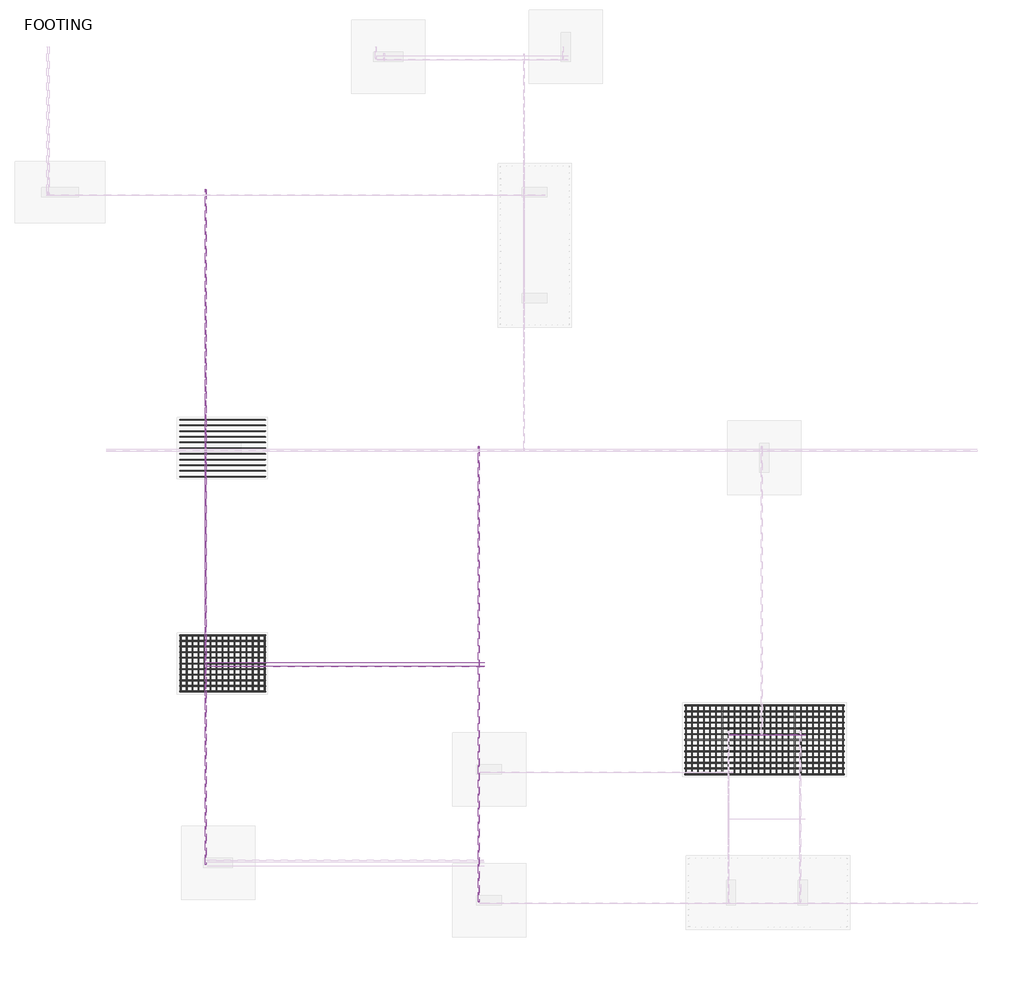
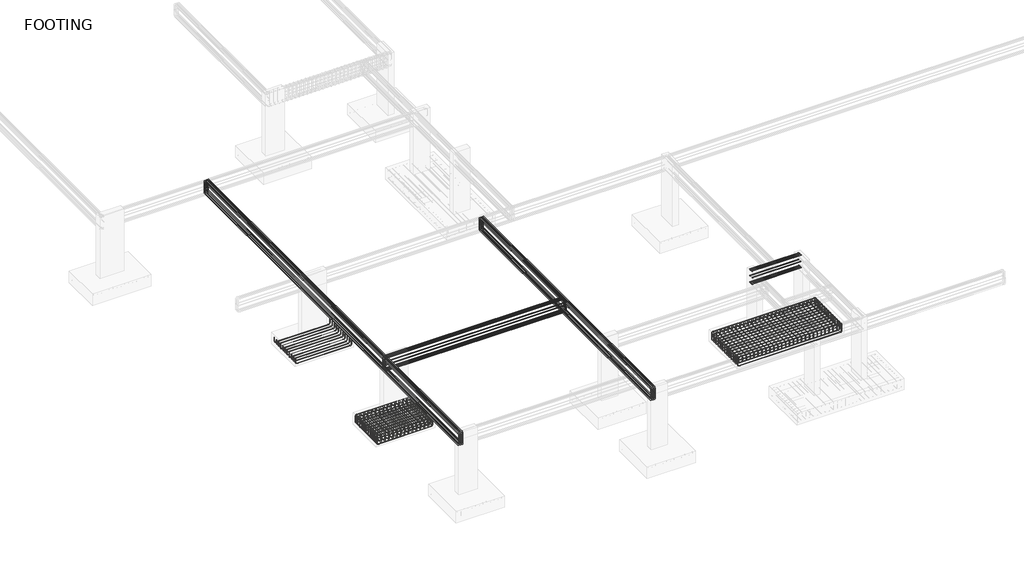
# One storey, part 4 of 12: 20 reinforcing bars.
"""IFC4 building model written with IfcOpenShell, lengths in millimetres."""

from ifc_helpers import new_model, si_unit, point, frame, origin, place, context, project, spatial, polyline, circle_curve, trimmed, segment, composite_curve, source, transform, mapped, element, save
from ifc_brep_helpers import swept_disk

model = new_model("IFC4")

# Units and contexts
model_context = context("Model", 3, world=origin())
ifc_project = project(units=[si_unit("LENGTHUNIT", "METRE", prefix="MILLI")], contexts=[model_context])

# Site, building, storey
site = spatial("IfcSite", under=ifc_project)
building = spatial("IfcBuilding", under=site)
storey = spatial("IfcBuildingStorey", under=building, Name="FOOTING", Elevation=-5638.8)

# Reinforcing bars
placement = place(None, origin())
reinforcing_bar_shape = source(origin(), model_context, "Body", "SolidModel", [
    swept_disk(composite_curve([segment(polyline([(209.0067827, -8447.9541655, -5901.65), (209.0067827, -8447.9541655, -5754.35)]), True, "CONTINUOUS"), segment(trimmed(circle_curve(frame((209.0067827, -8494.3041655, -5754.35), z_axis=(1.0, 0.0, 0.0), x_axis=(0.0, 46.350000000000364, 0.0)), 46.35), [point((209.0067827, -8447.9541655, -5754.35))], [point((209.0067827, -8494.3041655, -5708.0))], True, "CARTESIAN"), True, "CONTINUOUS"), segment(polyline([(209.0067827, -8494.3041655, -5708.0), (209.0067827, -10088.9041655, -5708.0)]), True, "CONTINUOUS"), segment(trimmed(circle_curve(frame((209.0067827, -10088.9041655, -5754.35), z_axis=(1.0, 0.0, 0.0), x_axis=(0.0, 0.0, 46.350000000000364)), 46.35), [point((209.0067827, -10088.9041655, -5708.0))], [point((209.0067827, -10135.2541655, -5754.35))], True, "CARTESIAN"), True, "CONTINUOUS"), segment(polyline([(209.0067827, -10135.2541655, -5754.35), (209.0067827, -10135.2541655, -5901.65)]), True, "CONTINUOUS")], self_intersect=False), 6.35),
])
element("IfcReinforcingBar", 1, at=placement, inside=storey, context=model_context, shape_type="MappedRepresentation", body=[
    mapped(reinforcing_bar_shape, transform((0.0, 0.0, 0.0), x_axis=(1.0, 0.0, 0.0), y_axis=(0.0, 1.0, 0.0), z_axis=(0.0, 0.0, 1.0))),
    mapped(reinforcing_bar_shape, transform((-147.4810365, 0.0, 0.0), x_axis=(1.0, 0.0, 0.0), y_axis=(0.0, 1.0, 0.0), z_axis=(0.0, 0.0, 1.0))),
    mapped(reinforcing_bar_shape, transform((-294.962073, 0.0, 0.0), x_axis=(1.0, 0.0, 0.0), y_axis=(0.0, 1.0, 0.0), z_axis=(0.0, 0.0, 1.0))),
    mapped(reinforcing_bar_shape, transform((-442.4431095, 0.0, 0.0), x_axis=(1.0, 0.0, 0.0), y_axis=(0.0, 1.0, 0.0), z_axis=(0.0, 0.0, 1.0))),
    mapped(reinforcing_bar_shape, transform((-589.924146, 0.0, 0.0), x_axis=(1.0, 0.0, 0.0), y_axis=(0.0, 1.0, 0.0), z_axis=(0.0, 0.0, 1.0))),
    mapped(reinforcing_bar_shape, transform((-737.4051825, 0.0, 0.0), x_axis=(1.0, 0.0, 0.0), y_axis=(0.0, 1.0, 0.0), z_axis=(0.0, 0.0, 1.0))),
    mapped(reinforcing_bar_shape, transform((-884.886219, 0.0, 0.0), x_axis=(1.0, 0.0, 0.0), y_axis=(0.0, 1.0, 0.0), z_axis=(0.0, 0.0, 1.0))),
    mapped(reinforcing_bar_shape, transform((-1032.3672556, 0.0, 0.0), x_axis=(1.0, 0.0, 0.0), y_axis=(0.0, 1.0, 0.0), z_axis=(0.0, 0.0, 1.0))),
    mapped(reinforcing_bar_shape, transform((-1179.8482921, 0.0, 0.0), x_axis=(1.0, 0.0, 0.0), y_axis=(0.0, 1.0, 0.0), z_axis=(0.0, 0.0, 1.0))),
    mapped(reinforcing_bar_shape, transform((-1327.3293286, 0.0, 0.0), x_axis=(1.0, 0.0, 0.0), y_axis=(0.0, 1.0, 0.0), z_axis=(0.0, 0.0, 1.0))),
    mapped(reinforcing_bar_shape, transform((-1474.8103651, 0.0, 0.0), x_axis=(1.0, 0.0, 0.0), y_axis=(0.0, 1.0, 0.0), z_axis=(0.0, 0.0, 1.0))),
    mapped(reinforcing_bar_shape, transform((-1622.2914016, 0.0, 0.0), x_axis=(1.0, 0.0, 0.0), y_axis=(0.0, 1.0, 0.0), z_axis=(0.0, 0.0, 1.0))),
    mapped(reinforcing_bar_shape, transform((-1769.7724381, 0.0, 0.0), x_axis=(1.0, 0.0, 0.0), y_axis=(0.0, 1.0, 0.0), z_axis=(0.0, 0.0, 1.0))),
    mapped(reinforcing_bar_shape, transform((-1917.2534746, 0.0, 0.0), x_axis=(1.0, 0.0, 0.0), y_axis=(0.0, 1.0, 0.0), z_axis=(0.0, 0.0, 1.0))),
    mapped(reinforcing_bar_shape, transform((-2064.7345111, 0.0, 0.0), x_axis=(1.0, 0.0, 0.0), y_axis=(0.0, 1.0, 0.0), z_axis=(0.0, 0.0, 1.0))),
    mapped(reinforcing_bar_shape, transform((-2212.2155476, 0.0, 0.0), x_axis=(1.0, 0.0, 0.0), y_axis=(0.0, 1.0, 0.0), z_axis=(0.0, 0.0, 1.0))),
    mapped(reinforcing_bar_shape, transform((-2359.6965841, 0.0, 0.0), x_axis=(1.0, 0.0, 0.0), y_axis=(0.0, 1.0, 0.0), z_axis=(0.0, 0.0, 1.0))),
    mapped(reinforcing_bar_shape, transform((-2507.1776206, 0.0, 0.0), x_axis=(1.0, 0.0, 0.0), y_axis=(0.0, 1.0, 0.0), z_axis=(0.0, 0.0, 1.0))),
    mapped(reinforcing_bar_shape, transform((-2654.6586571, 0.0, 0.0), x_axis=(1.0, 0.0, 0.0), y_axis=(0.0, 1.0, 0.0), z_axis=(0.0, 0.0, 1.0))),
    mapped(reinforcing_bar_shape, transform((-2802.1396936, 0.0, 0.0), x_axis=(1.0, 0.0, 0.0), y_axis=(0.0, 1.0, 0.0), z_axis=(0.0, 0.0, 1.0))),
    mapped(reinforcing_bar_shape, transform((-2949.6207301, 0.0, 0.0), x_axis=(1.0, 0.0, 0.0), y_axis=(0.0, 1.0, 0.0), z_axis=(0.0, 0.0, 1.0))),
    mapped(reinforcing_bar_shape, transform((-3097.1017667, 0.0, 0.0), x_axis=(1.0, 0.0, 0.0), y_axis=(0.0, 1.0, 0.0), z_axis=(0.0, 0.0, 1.0))),
    mapped(reinforcing_bar_shape, transform((-3244.5828032, 0.0, 0.0), x_axis=(1.0, 0.0, 0.0), y_axis=(0.0, 1.0, 0.0), z_axis=(0.0, 0.0, 1.0))),
    mapped(reinforcing_bar_shape, transform((-3392.0638397, 0.0, 0.0), x_axis=(1.0, 0.0, 0.0), y_axis=(0.0, 1.0, 0.0), z_axis=(0.0, 0.0, 1.0))),
    mapped(reinforcing_bar_shape, transform((-3539.5448762, 0.0, 0.0), x_axis=(1.0, 0.0, 0.0), y_axis=(0.0, 1.0, 0.0), z_axis=(0.0, 0.0, 1.0))),
    mapped(reinforcing_bar_shape, transform((-3687.0259127, 0.0, 0.0), x_axis=(1.0, 0.0, 0.0), y_axis=(0.0, 1.0, 0.0), z_axis=(0.0, 0.0, 1.0))),
    mapped(reinforcing_bar_shape, transform((-3834.5069492, 0.0, 0.0), x_axis=(1.0, 0.0, 0.0), y_axis=(0.0, 1.0, 0.0), z_axis=(0.0, 0.0, 1.0))),
])
reinforcing_bar_2_shape = source(origin(), model_context, "Body", "SolidModel", [
    swept_disk(composite_curve([segment(polyline([(-3650.5001665, -10135.2541655, -5838.8), (-3650.5001665, -10135.2541655, -5986.1)]), True, "CONTINUOUS"), segment(trimmed(circle_curve(frame((-3604.1501665, -10135.2541655, -5986.1), z_axis=(0.0, -1.0, 0.0), x_axis=(-46.34999999999991, 0.0, 0.0)), 46.35), [point((-3650.5001665, -10135.2541655, -5986.1))], [point((-3604.1501665, -10135.2541655, -6032.45))], True, "CARTESIAN"), True, "CONTINUOUS"), segment(polyline([(-3604.1501665, -10135.2541655, -6032.45), (190.4498335, -10135.2541655, -6032.45)]), True, "CONTINUOUS"), segment(trimmed(circle_curve(frame((190.4498335, -10135.2541655, -5986.1), z_axis=(0.0, -1.0, 0.0), x_axis=(0.0, 0.0, -46.349999999999454)), 46.35), [point((190.4498335, -10135.2541655, -6032.45))], [point((236.7998335, -10135.2541655, -5986.1))], True, "CARTESIAN"), True, "CONTINUOUS"), segment(polyline([(236.7998335, -10135.2541655, -5986.1), (236.7998335, -10135.2541655, -5838.8)]), True, "CONTINUOUS")], self_intersect=False), 6.35),
])
element("IfcReinforcingBar", 2, at=placement, inside=storey, context=model_context, shape_type="MappedRepresentation", body=[
    mapped(reinforcing_bar_2_shape, transform((0.0, 0.0, 0.0), x_axis=(1.0, 0.0, 0.0), y_axis=(0.0, 1.0, 0.0), z_axis=(0.0, 0.0, 1.0))),
    mapped(reinforcing_bar_2_shape, transform((0.0, 140.6083333, 0.0), x_axis=(1.0, 0.0, 0.0), y_axis=(0.0, 1.0, 0.0), z_axis=(0.0, 0.0, 1.0))),
    mapped(reinforcing_bar_2_shape, transform((0.0, 281.2166667, 0.0), x_axis=(1.0, 0.0, 0.0), y_axis=(0.0, 1.0, 0.0), z_axis=(0.0, 0.0, 1.0))),
    mapped(reinforcing_bar_2_shape, transform((0.0, 421.825, 0.0), x_axis=(1.0, 0.0, 0.0), y_axis=(0.0, 1.0, 0.0), z_axis=(0.0, 0.0, 1.0))),
    mapped(reinforcing_bar_2_shape, transform((0.0, 562.4333333, 0.0), x_axis=(1.0, 0.0, 0.0), y_axis=(0.0, 1.0, 0.0), z_axis=(0.0, 0.0, 1.0))),
    mapped(reinforcing_bar_2_shape, transform((0.0, 703.0416667, 0.0), x_axis=(1.0, 0.0, 0.0), y_axis=(0.0, 1.0, 0.0), z_axis=(0.0, 0.0, 1.0))),
    mapped(reinforcing_bar_2_shape, transform((0.0, 843.65, 0.0), x_axis=(1.0, 0.0, 0.0), y_axis=(0.0, 1.0, 0.0), z_axis=(0.0, 0.0, 1.0))),
    mapped(reinforcing_bar_2_shape, transform((0.0, 984.2583333, 0.0), x_axis=(1.0, 0.0, 0.0), y_axis=(0.0, 1.0, 0.0), z_axis=(0.0, 0.0, 1.0))),
    mapped(reinforcing_bar_2_shape, transform((0.0, 1124.8666667, 0.0), x_axis=(1.0, 0.0, 0.0), y_axis=(0.0, 1.0, 0.0), z_axis=(0.0, 0.0, 1.0))),
    mapped(reinforcing_bar_2_shape, transform((0.0, 1265.475, 0.0), x_axis=(1.0, 0.0, 0.0), y_axis=(0.0, 1.0, 0.0), z_axis=(0.0, 0.0, 1.0))),
    mapped(reinforcing_bar_2_shape, transform((0.0, 1406.0833333, 0.0), x_axis=(1.0, 0.0, 0.0), y_axis=(0.0, 1.0, 0.0), z_axis=(0.0, 0.0, 1.0))),
    mapped(reinforcing_bar_2_shape, transform((0.0, 1546.6916667, 0.0), x_axis=(1.0, 0.0, 0.0), y_axis=(0.0, 1.0, 0.0), z_axis=(0.0, 0.0, 1.0))),
    mapped(reinforcing_bar_2_shape, transform((0.0, 1687.3, 0.0), x_axis=(1.0, 0.0, 0.0), y_axis=(0.0, 1.0, 0.0), z_axis=(0.0, 0.0, 1.0))),
])
reinforcing_bar_3_shape = source(origin(), model_context, "Body", "SolidModel", [
    swept_disk(composite_curve([segment(polyline([(236.7998335, -10122.5720387, -5888.8), (236.7998335, -10122.5720387, -5741.5)]), True, "CONTINUOUS"), segment(trimmed(circle_curve(frame((190.4498335, -10122.5720387, -5741.5), z_axis=(0.0, -1.0, 0.0), x_axis=(46.349999999999994, 0.0, 0.0)), 46.35), [point((236.7998335, -10122.5720387, -5741.5))], [point((190.4498335, -10122.5720387, -5695.15))], True, "CARTESIAN"), True, "CONTINUOUS"), segment(polyline([(190.4498335, -10122.5720387, -5695.15), (-3604.1501665, -10122.5720387, -5695.15)]), True, "CONTINUOUS"), segment(trimmed(circle_curve(frame((-3604.1501665, -10122.5720387, -5741.5), z_axis=(0.0, -1.0, 0.0), x_axis=(0.0, 0.0, 46.350000000000364)), 46.35), [point((-3604.1501665, -10122.5720387, -5695.15))], [point((-3650.5001665, -10122.5720387, -5741.5))], True, "CARTESIAN"), True, "CONTINUOUS"), segment(polyline([(-3650.5001665, -10122.5720387, -5741.5), (-3650.5001665, -10122.5720387, -5888.8)]), True, "CONTINUOUS")], self_intersect=False), 6.35),
])
element("IfcReinforcingBar", 3, at=placement, inside=storey, context=model_context, shape_type="MappedRepresentation", body=[
    mapped(reinforcing_bar_3_shape, transform((0.0, 0.0, 0.0), x_axis=(1.0, 0.0, 0.0), y_axis=(0.0, 1.0, 0.0), z_axis=(0.0, 0.0, 1.0))),
    mapped(reinforcing_bar_3_shape, transform((0.0, 138.5098228, 0.0), x_axis=(1.0, 0.0, 0.0), y_axis=(0.0, 1.0, 0.0), z_axis=(0.0, 0.0, 1.0))),
    mapped(reinforcing_bar_3_shape, transform((0.0, 277.0196455, 0.0), x_axis=(1.0, 0.0, 0.0), y_axis=(0.0, 1.0, 0.0), z_axis=(0.0, 0.0, 1.0))),
    mapped(reinforcing_bar_3_shape, transform((0.0, 415.5294683, 0.0), x_axis=(1.0, 0.0, 0.0), y_axis=(0.0, 1.0, 0.0), z_axis=(0.0, 0.0, 1.0))),
    mapped(reinforcing_bar_3_shape, transform((0.0, 554.0392911, 0.0), x_axis=(1.0, 0.0, 0.0), y_axis=(0.0, 1.0, 0.0), z_axis=(0.0, 0.0, 1.0))),
    mapped(reinforcing_bar_3_shape, transform((0.0, 692.5491138, 0.0), x_axis=(1.0, 0.0, 0.0), y_axis=(0.0, 1.0, 0.0), z_axis=(0.0, 0.0, 1.0))),
    mapped(reinforcing_bar_3_shape, transform((0.0, 831.0589366, 0.0), x_axis=(1.0, 0.0, 0.0), y_axis=(0.0, 1.0, 0.0), z_axis=(0.0, 0.0, 1.0))),
    mapped(reinforcing_bar_3_shape, transform((0.0, 969.5687594, 0.0), x_axis=(1.0, 0.0, 0.0), y_axis=(0.0, 1.0, 0.0), z_axis=(0.0, 0.0, 1.0))),
    mapped(reinforcing_bar_3_shape, transform((0.0, 1108.0785821, 0.0), x_axis=(1.0, 0.0, 0.0), y_axis=(0.0, 1.0, 0.0), z_axis=(0.0, 0.0, 1.0))),
    mapped(reinforcing_bar_3_shape, transform((0.0, 1246.5884049, 0.0), x_axis=(1.0, 0.0, 0.0), y_axis=(0.0, 1.0, 0.0), z_axis=(0.0, 0.0, 1.0))),
    mapped(reinforcing_bar_3_shape, transform((0.0, 1385.0982277, 0.0), x_axis=(1.0, 0.0, 0.0), y_axis=(0.0, 1.0, 0.0), z_axis=(0.0, 0.0, 1.0))),
    mapped(reinforcing_bar_3_shape, transform((0.0, 1523.6080504, 0.0), x_axis=(1.0, 0.0, 0.0), y_axis=(0.0, 1.0, 0.0), z_axis=(0.0, 0.0, 1.0))),
    mapped(reinforcing_bar_3_shape, transform((0.0, 1662.1178732, 0.0), x_axis=(1.0, 0.0, 0.0), y_axis=(0.0, 1.0, 0.0), z_axis=(0.0, 0.0, 1.0))),
])
reinforcing_bar_4_shape = source(origin(), model_context, "Body", "SolidModel", [
    swept_disk(composite_curve([segment(polyline([(-15983.9001665, -8118.3541655, -5837.6659404), (-15983.9001665, -8118.3541655, -5984.9659404)]), True, "CONTINUOUS"), segment(trimmed(circle_curve(frame((-15937.5501665, -8118.3541655, -5984.9659404), z_axis=(0.0, -1.0, 0.0), x_axis=(-46.350000000000364, 0.0, 0.0)), 46.35), [point((-15983.9001665, -8118.3541655, -5984.9659404))], [point((-15937.5501665, -8118.3541655, -6031.3159404))], True, "CARTESIAN"), True, "CONTINUOUS"), segment(polyline([(-15937.5501665, -8118.3541655, -6031.3159404), (-13942.9501665, -8118.3541655, -6031.3159404)]), True, "CONTINUOUS"), segment(trimmed(circle_curve(frame((-13942.9501665, -8118.3541655, -5984.9659404), z_axis=(0.0, -1.0, 0.0), x_axis=(0.0, 0.0, -46.349999999999454)), 46.35), [point((-13942.9501665, -8118.3541655, -6031.3159404))], [point((-13896.6001665, -8118.3541655, -5984.9659404))], True, "CARTESIAN"), True, "CONTINUOUS"), segment(polyline([(-13896.6001665, -8118.3541655, -5984.9659404), (-13896.6001665, -8118.3541655, -5837.6659404)]), True, "CONTINUOUS")], self_intersect=False), 6.35),
])
element("IfcReinforcingBar", 4, at=placement, inside=storey, context=model_context, shape_type="MappedRepresentation", body=[
    mapped(reinforcing_bar_4_shape, transform((0.0, 0.0, 0.0), x_axis=(1.0, 0.0, 0.0), y_axis=(0.0, 1.0, 0.0), z_axis=(0.0, 0.0, 1.0))),
    mapped(reinforcing_bar_4_shape, transform((0.0, 138.73, 0.0), x_axis=(1.0, 0.0, 0.0), y_axis=(0.0, 1.0, 0.0), z_axis=(0.0, 0.0, 1.0))),
    mapped(reinforcing_bar_4_shape, transform((0.0, 277.46, 0.0), x_axis=(1.0, 0.0, 0.0), y_axis=(0.0, 1.0, 0.0), z_axis=(0.0, 0.0, 1.0))),
    mapped(reinforcing_bar_4_shape, transform((0.0, 416.19, 0.0), x_axis=(1.0, 0.0, 0.0), y_axis=(0.0, 1.0, 0.0), z_axis=(0.0, 0.0, 1.0))),
    mapped(reinforcing_bar_4_shape, transform((0.0, 554.92, 0.0), x_axis=(1.0, 0.0, 0.0), y_axis=(0.0, 1.0, 0.0), z_axis=(0.0, 0.0, 1.0))),
    mapped(reinforcing_bar_4_shape, transform((0.0, 693.65, 0.0), x_axis=(1.0, 0.0, 0.0), y_axis=(0.0, 1.0, 0.0), z_axis=(0.0, 0.0, 1.0))),
    mapped(reinforcing_bar_4_shape, transform((0.0, 832.38, 0.0), x_axis=(1.0, 0.0, 0.0), y_axis=(0.0, 1.0, 0.0), z_axis=(0.0, 0.0, 1.0))),
    mapped(reinforcing_bar_4_shape, transform((0.0, 971.11, 0.0), x_axis=(1.0, 0.0, 0.0), y_axis=(0.0, 1.0, 0.0), z_axis=(0.0, 0.0, 1.0))),
    mapped(reinforcing_bar_4_shape, transform((0.0, 1109.84, 0.0), x_axis=(1.0, 0.0, 0.0), y_axis=(0.0, 1.0, 0.0), z_axis=(0.0, 0.0, 1.0))),
    mapped(reinforcing_bar_4_shape, transform((0.0, 1248.57, 0.0), x_axis=(1.0, 0.0, 0.0), y_axis=(0.0, 1.0, 0.0), z_axis=(0.0, 0.0, 1.0))),
    mapped(reinforcing_bar_4_shape, transform((0.0, 1387.3, 0.0), x_axis=(1.0, 0.0, 0.0), y_axis=(0.0, 1.0, 0.0), z_axis=(0.0, 0.0, 1.0))),
])
reinforcing_bar_5_shape = source(origin(), model_context, "Body", "SolidModel", [
    swept_disk(composite_curve([segment(polyline([(-13896.6001665, -8105.5545193, -5888.8), (-13896.6001665, -8105.5545193, -5741.5)]), True, "CONTINUOUS"), segment(trimmed(circle_curve(frame((-13942.9501665, -8105.5545193, -5741.5), z_axis=(0.0, -1.0, 0.0), x_axis=(46.350000000000364, 0.0, 0.0)), 46.35), [point((-13896.6001665, -8105.5545193, -5741.5))], [point((-13942.9501665, -8105.5545193, -5695.15))], True, "CARTESIAN"), True, "CONTINUOUS"), segment(polyline([(-13942.9501665, -8105.5545193, -5695.15), (-15937.5501665, -8105.5545193, -5695.15)]), True, "CONTINUOUS"), segment(trimmed(circle_curve(frame((-15937.5501665, -8105.5545193, -5741.5), z_axis=(0.0, -1.0, 0.0), x_axis=(0.0, 0.0, 46.350000000000364)), 46.35), [point((-15937.5501665, -8105.5545193, -5695.15))], [point((-15983.9001665, -8105.5545193, -5741.5))], True, "CARTESIAN"), True, "CONTINUOUS"), segment(polyline([(-15983.9001665, -8105.5545193, -5741.5), (-15983.9001665, -8105.5545193, -5888.8)]), True, "CONTINUOUS")], self_intersect=False), 6.35),
])
element("IfcReinforcingBar", 5, at=placement, inside=storey, context=model_context, shape_type="MappedRepresentation", body=[
    mapped(reinforcing_bar_5_shape, transform((0.0, 0.0, 0.0), x_axis=(1.0, 0.0, 0.0), y_axis=(0.0, 1.0, 0.0), z_axis=(0.0, 0.0, 1.0))),
    mapped(reinforcing_bar_5_shape, transform((0.0, 136.1586067, 0.0), x_axis=(1.0, 0.0, 0.0), y_axis=(0.0, 1.0, 0.0), z_axis=(0.0, 0.0, 1.0))),
    mapped(reinforcing_bar_5_shape, transform((0.0, 272.3172133, 0.0), x_axis=(1.0, 0.0, 0.0), y_axis=(0.0, 1.0, 0.0), z_axis=(0.0, 0.0, 1.0))),
    mapped(reinforcing_bar_5_shape, transform((0.0, 408.47582, 0.0), x_axis=(1.0, 0.0, 0.0), y_axis=(0.0, 1.0, 0.0), z_axis=(0.0, 0.0, 1.0))),
    mapped(reinforcing_bar_5_shape, transform((0.0, 544.6344267, 0.0), x_axis=(1.0, 0.0, 0.0), y_axis=(0.0, 1.0, 0.0), z_axis=(0.0, 0.0, 1.0))),
    mapped(reinforcing_bar_5_shape, transform((0.0, 680.7930333, 0.0), x_axis=(1.0, 0.0, 0.0), y_axis=(0.0, 1.0, 0.0), z_axis=(0.0, 0.0, 1.0))),
    mapped(reinforcing_bar_5_shape, transform((0.0, 816.95164, 0.0), x_axis=(1.0, 0.0, 0.0), y_axis=(0.0, 1.0, 0.0), z_axis=(0.0, 0.0, 1.0))),
    mapped(reinforcing_bar_5_shape, transform((0.0, 953.1102467, 0.0), x_axis=(1.0, 0.0, 0.0), y_axis=(0.0, 1.0, 0.0), z_axis=(0.0, 0.0, 1.0))),
    mapped(reinforcing_bar_5_shape, transform((0.0, 1089.2688533, 0.0), x_axis=(1.0, 0.0, 0.0), y_axis=(0.0, 1.0, 0.0), z_axis=(0.0, 0.0, 1.0))),
    mapped(reinforcing_bar_5_shape, transform((0.0, 1225.42746, 0.0), x_axis=(1.0, 0.0, 0.0), y_axis=(0.0, 1.0, 0.0), z_axis=(0.0, 0.0, 1.0))),
    mapped(reinforcing_bar_5_shape, transform((0.0, 1361.5860667, 0.0), x_axis=(1.0, 0.0, 0.0), y_axis=(0.0, 1.0, 0.0), z_axis=(0.0, 0.0, 1.0))),
])
reinforcing_bar_6_shape = source(origin(), model_context, "Body", "SolidModel", [
    swept_disk(composite_curve([segment(polyline([(-15971.9866414, -6731.0541655, -5821.490176), (-15971.9866414, -6731.0541655, -5968.790176)]), True, "CONTINUOUS"), segment(trimmed(circle_curve(frame((-15971.9866414, -6777.4041655, -5968.790176), z_axis=(-1.0, 0.0, 0.0), x_axis=(0.0, 46.350000000000364, 0.0)), 46.35), [point((-15971.9866414, -6731.0541655, -5968.790176))], [point((-15971.9866414, -6777.4041655, -6015.140176))], True, "CARTESIAN"), True, "CONTINUOUS"), segment(polyline([(-15971.9866414, -6777.4041655, -6015.140176), (-15971.9866414, -8072.0041655, -6015.140176)]), True, "CONTINUOUS"), segment(trimmed(circle_curve(frame((-15971.9866414, -8072.0041655, -5968.790176), z_axis=(-1.0, 0.0, 0.0), x_axis=(0.0, 0.0, -46.349999999999454)), 46.35), [point((-15971.9866414, -8072.0041655, -6015.140176))], [point((-15971.9866414, -8118.3541655, -5968.790176))], True, "CARTESIAN"), True, "CONTINUOUS"), segment(polyline([(-15971.9866414, -8118.3541655, -5968.790176), (-15971.9866414, -8118.3541655, -5821.490176)]), True, "CONTINUOUS")], self_intersect=False), 6.35),
])
element("IfcReinforcingBar", 6, at=placement, inside=storey, context=model_context, shape_type="MappedRepresentation", body=[
    mapped(reinforcing_bar_6_shape, transform((0.0, 0.0, 0.0), x_axis=(1.0, 0.0, 0.0), y_axis=(0.0, 1.0, 0.0), z_axis=(0.0, 0.0, 1.0))),
    mapped(reinforcing_bar_6_shape, transform((147.43641, 0.0, 0.0), x_axis=(1.0, 0.0, 0.0), y_axis=(0.0, 1.0, 0.0), z_axis=(0.0, 0.0, 1.0))),
    mapped(reinforcing_bar_6_shape, transform((294.87282, 0.0, 0.0), x_axis=(1.0, 0.0, 0.0), y_axis=(0.0, 1.0, 0.0), z_axis=(0.0, 0.0, 1.0))),
    mapped(reinforcing_bar_6_shape, transform((442.30923, 0.0, 0.0), x_axis=(1.0, 0.0, 0.0), y_axis=(0.0, 1.0, 0.0), z_axis=(0.0, 0.0, 1.0))),
    mapped(reinforcing_bar_6_shape, transform((589.74564, 0.0, 0.0), x_axis=(1.0, 0.0, 0.0), y_axis=(0.0, 1.0, 0.0), z_axis=(0.0, 0.0, 1.0))),
    mapped(reinforcing_bar_6_shape, transform((737.1820499, 0.0, 0.0), x_axis=(1.0, 0.0, 0.0), y_axis=(0.0, 1.0, 0.0), z_axis=(0.0, 0.0, 1.0))),
    mapped(reinforcing_bar_6_shape, transform((884.6184599, 0.0, 0.0), x_axis=(1.0, 0.0, 0.0), y_axis=(0.0, 1.0, 0.0), z_axis=(0.0, 0.0, 1.0))),
    mapped(reinforcing_bar_6_shape, transform((1032.0548699, 0.0, 0.0), x_axis=(1.0, 0.0, 0.0), y_axis=(0.0, 1.0, 0.0), z_axis=(0.0, 0.0, 1.0))),
    mapped(reinforcing_bar_6_shape, transform((1179.4912799, 0.0, 0.0), x_axis=(1.0, 0.0, 0.0), y_axis=(0.0, 1.0, 0.0), z_axis=(0.0, 0.0, 1.0))),
    mapped(reinforcing_bar_6_shape, transform((1326.9276899, 0.0, 0.0), x_axis=(1.0, 0.0, 0.0), y_axis=(0.0, 1.0, 0.0), z_axis=(0.0, 0.0, 1.0))),
    mapped(reinforcing_bar_6_shape, transform((1474.3640999, 0.0, 0.0), x_axis=(1.0, 0.0, 0.0), y_axis=(0.0, 1.0, 0.0), z_axis=(0.0, 0.0, 1.0))),
    mapped(reinforcing_bar_6_shape, transform((1621.8005099, 0.0, 0.0), x_axis=(1.0, 0.0, 0.0), y_axis=(0.0, 1.0, 0.0), z_axis=(0.0, 0.0, 1.0))),
    mapped(reinforcing_bar_6_shape, transform((1769.2369199, 0.0, 0.0), x_axis=(1.0, 0.0, 0.0), y_axis=(0.0, 1.0, 0.0), z_axis=(0.0, 0.0, 1.0))),
    mapped(reinforcing_bar_6_shape, transform((1916.6733299, 0.0, 0.0), x_axis=(1.0, 0.0, 0.0), y_axis=(0.0, 1.0, 0.0), z_axis=(0.0, 0.0, 1.0))),
    mapped(reinforcing_bar_6_shape, transform((2064.1097398, 0.0, 0.0), x_axis=(1.0, 0.0, 0.0), y_axis=(0.0, 1.0, 0.0), z_axis=(0.0, 0.0, 1.0))),
])
reinforcing_bar_7_shape = source(origin(), model_context, "Body", "SolidModel", [
    swept_disk(composite_curve([segment(polyline([(-13921.5742888, -6731.0541655, -5898.1017616), (-13921.5742888, -6731.0541655, -5750.8017616)]), True, "CONTINUOUS"), segment(trimmed(circle_curve(frame((-13921.5742888, -6777.4041655, -5750.8017616), z_axis=(1.0, 0.0, 0.0), x_axis=(0.0, 46.350000000000364, 0.0)), 46.35), [point((-13921.5742888, -6731.0541655, -5750.8017616))], [point((-13921.5742888, -6777.4041655, -5704.4517616))], True, "CARTESIAN"), True, "CONTINUOUS"), segment(polyline([(-13921.5742888, -6777.4041655, -5704.4517616), (-13921.5742888, -8072.0041655, -5704.4517616)]), True, "CONTINUOUS"), segment(trimmed(circle_curve(frame((-13921.5742888, -8072.0041655, -5750.8017616), z_axis=(1.0, 0.0, 0.0), x_axis=(0.0, 0.0, 46.349999999999454)), 46.35), [point((-13921.5742888, -8072.0041655, -5704.4517616))], [point((-13921.5742888, -8118.3541655, -5750.8017616))], True, "CARTESIAN"), True, "CONTINUOUS"), segment(polyline([(-13921.5742888, -8118.3541655, -5750.8017616), (-13921.5742888, -8118.3541655, -5898.1017616)]), True, "CONTINUOUS")], self_intersect=False), 6.35),
])
element("IfcReinforcingBar", 7, at=placement, inside=storey, context=model_context, shape_type="MappedRepresentation", body=[
    mapped(reinforcing_bar_7_shape, transform((0.0, 0.0, 0.0), x_axis=(1.0, 0.0, 0.0), y_axis=(0.0, 1.0, 0.0), z_axis=(0.0, 0.0, 1.0))),
    mapped(reinforcing_bar_7_shape, transform((-145.5195783, 0.0, 0.0), x_axis=(1.0, 0.0, 0.0), y_axis=(0.0, 1.0, 0.0), z_axis=(0.0, 0.0, 1.0))),
    mapped(reinforcing_bar_7_shape, transform((-291.0391566, 0.0, 0.0), x_axis=(1.0, 0.0, 0.0), y_axis=(0.0, 1.0, 0.0), z_axis=(0.0, 0.0, 1.0))),
    mapped(reinforcing_bar_7_shape, transform((-436.5587348, 0.0, 0.0), x_axis=(1.0, 0.0, 0.0), y_axis=(0.0, 1.0, 0.0), z_axis=(0.0, 0.0, 1.0))),
    mapped(reinforcing_bar_7_shape, transform((-582.0783131, 0.0, 0.0), x_axis=(1.0, 0.0, 0.0), y_axis=(0.0, 1.0, 0.0), z_axis=(0.0, 0.0, 1.0))),
    mapped(reinforcing_bar_7_shape, transform((-727.5978914, 0.0, 0.0), x_axis=(1.0, 0.0, 0.0), y_axis=(0.0, 1.0, 0.0), z_axis=(0.0, 0.0, 1.0))),
    mapped(reinforcing_bar_7_shape, transform((-873.1174697, 0.0, 0.0), x_axis=(1.0, 0.0, 0.0), y_axis=(0.0, 1.0, 0.0), z_axis=(0.0, 0.0, 1.0))),
    mapped(reinforcing_bar_7_shape, transform((-1018.637048, 0.0, 0.0), x_axis=(1.0, 0.0, 0.0), y_axis=(0.0, 1.0, 0.0), z_axis=(0.0, 0.0, 1.0))),
    mapped(reinforcing_bar_7_shape, transform((-1164.1566263, 0.0, 0.0), x_axis=(1.0, 0.0, 0.0), y_axis=(0.0, 1.0, 0.0), z_axis=(0.0, 0.0, 1.0))),
    mapped(reinforcing_bar_7_shape, transform((-1309.6762045, 0.0, 0.0), x_axis=(1.0, 0.0, 0.0), y_axis=(0.0, 1.0, 0.0), z_axis=(0.0, 0.0, 1.0))),
    mapped(reinforcing_bar_7_shape, transform((-1455.1957828, 0.0, 0.0), x_axis=(1.0, 0.0, 0.0), y_axis=(0.0, 1.0, 0.0), z_axis=(0.0, 0.0, 1.0))),
    mapped(reinforcing_bar_7_shape, transform((-1600.7153611, 0.0, 0.0), x_axis=(1.0, 0.0, 0.0), y_axis=(0.0, 1.0, 0.0), z_axis=(0.0, 0.0, 1.0))),
    mapped(reinforcing_bar_7_shape, transform((-1746.2349394, 0.0, 0.0), x_axis=(1.0, 0.0, 0.0), y_axis=(0.0, 1.0, 0.0), z_axis=(0.0, 0.0, 1.0))),
    mapped(reinforcing_bar_7_shape, transform((-1891.7545177, 0.0, 0.0), x_axis=(1.0, 0.0, 0.0), y_axis=(0.0, 1.0, 0.0), z_axis=(0.0, 0.0, 1.0))),
    mapped(reinforcing_bar_7_shape, transform((-2037.2740959, 0.0, 0.0), x_axis=(1.0, 0.0, 0.0), y_axis=(0.0, 1.0, 0.0), z_axis=(0.0, 0.0, 1.0))),
])
reinforcing_bar_8_shape = source(origin(), model_context, "Body", "SolidModel", [
    swept_disk(composite_curve([segment(polyline([(-15983.9001665, -2860.5541655, -5837.6659404), (-15983.9001665, -2860.5541655, -5984.9659404)]), True, "CONTINUOUS"), segment(trimmed(circle_curve(frame((-15937.5501665, -2860.5541655, -5984.9659404), z_axis=(0.0, -1.0, 0.0), x_axis=(-46.350000000000364, 0.0, 0.0)), 46.35), [point((-15983.9001665, -2860.5541655, -5984.9659404))], [point((-15937.5501665, -2860.5541655, -6031.3159404))], True, "CARTESIAN"), True, "CONTINUOUS"), segment(polyline([(-15937.5501665, -2860.5541655, -6031.3159404), (-13942.9501665, -2860.5541655, -6031.3159404)]), True, "CONTINUOUS"), segment(trimmed(circle_curve(frame((-13942.9501665, -2860.5541655, -5984.9659404), z_axis=(0.0, -1.0, 0.0), x_axis=(0.0, 0.0, -46.349999999999454)), 46.35), [point((-13942.9501665, -2860.5541655, -6031.3159404))], [point((-13896.6001665, -2860.5541655, -5984.9659404))], True, "CARTESIAN"), True, "CONTINUOUS"), segment(polyline([(-13896.6001665, -2860.5541655, -5984.9659404), (-13896.6001665, -2860.5541655, -5837.6659404)]), True, "CONTINUOUS")], self_intersect=False), 6.35),
])
element("IfcReinforcingBar", 8, at=placement, inside=storey, context=model_context, shape_type="MappedRepresentation", body=[
    mapped(reinforcing_bar_8_shape, transform((0.0, 0.0, 0.0), x_axis=(1.0, 0.0, 0.0), y_axis=(0.0, 1.0, 0.0), z_axis=(0.0, 0.0, 1.0))),
    mapped(reinforcing_bar_8_shape, transform((0.0, 138.73, 0.0), x_axis=(1.0, 0.0, 0.0), y_axis=(0.0, 1.0, 0.0), z_axis=(0.0, 0.0, 1.0))),
    mapped(reinforcing_bar_8_shape, transform((0.0, 277.46, 0.0), x_axis=(1.0, 0.0, 0.0), y_axis=(0.0, 1.0, 0.0), z_axis=(0.0, 0.0, 1.0))),
    mapped(reinforcing_bar_8_shape, transform((0.0, 416.19, 0.0), x_axis=(1.0, 0.0, 0.0), y_axis=(0.0, 1.0, 0.0), z_axis=(0.0, 0.0, 1.0))),
    mapped(reinforcing_bar_8_shape, transform((0.0, 554.92, 0.0), x_axis=(1.0, 0.0, 0.0), y_axis=(0.0, 1.0, 0.0), z_axis=(0.0, 0.0, 1.0))),
    mapped(reinforcing_bar_8_shape, transform((0.0, 693.65, 0.0), x_axis=(1.0, 0.0, 0.0), y_axis=(0.0, 1.0, 0.0), z_axis=(0.0, 0.0, 1.0))),
    mapped(reinforcing_bar_8_shape, transform((0.0, 832.38, 0.0), x_axis=(1.0, 0.0, 0.0), y_axis=(0.0, 1.0, 0.0), z_axis=(0.0, 0.0, 1.0))),
    mapped(reinforcing_bar_8_shape, transform((0.0, 971.11, 0.0), x_axis=(1.0, 0.0, 0.0), y_axis=(0.0, 1.0, 0.0), z_axis=(0.0, 0.0, 1.0))),
    mapped(reinforcing_bar_8_shape, transform((0.0, 1109.84, 0.0), x_axis=(1.0, 0.0, 0.0), y_axis=(0.0, 1.0, 0.0), z_axis=(0.0, 0.0, 1.0))),
    mapped(reinforcing_bar_8_shape, transform((0.0, 1248.57, 0.0), x_axis=(1.0, 0.0, 0.0), y_axis=(0.0, 1.0, 0.0), z_axis=(0.0, 0.0, 1.0))),
    mapped(reinforcing_bar_8_shape, transform((0.0, 1387.3, 0.0), x_axis=(1.0, 0.0, 0.0), y_axis=(0.0, 1.0, 0.0), z_axis=(0.0, 0.0, 1.0))),
])
reinforcing_bar_9_shape = source(origin(), model_context, "Body", "SolidModel", [
    swept_disk(composite_curve([segment(polyline([(-8543.8001665, -13251.3307048, -3500.1457532), (-8543.8001665, -2115.7280815, -3500.1457532)]), True, "CONTINUOUS")], self_intersect=False), 7.95),
])
element("IfcReinforcingBar", 9, at=placement, inside=storey, context=model_context, shape_type="MappedRepresentation", body=[
    mapped(reinforcing_bar_9_shape, transform((0.0, 0.0, 0.0), x_axis=(1.0, 0.0, 0.0), y_axis=(0.0, 1.0, 0.0), z_axis=(0.0, 0.0, 1.0))),
    mapped(reinforcing_bar_9_shape, transform((-143.7, 0.0, 0.0), x_axis=(1.0, 0.0, 0.0), y_axis=(0.0, 1.0, 0.0), z_axis=(0.0, 0.0, 1.0))),
])
reinforcing_bar_10_shape = source(origin(), model_context, "Body", "SolidModel", [
    swept_disk(composite_curve([segment(polyline([(-8547.3295298, -13243.7204013, -3488.4293633), (-8547.3295298, -13243.7204013, -3301.8293633)]), True, "CONTINUOUS"), segment(trimmed(circle_curve(frame((-8547.3295298, -13188.2704013, -3301.8293633), z_axis=(-1.0, 0.0, 0.0), x_axis=(0.0, -55.44999999999891, 0.0)), 55.45), [point((-8547.3295298, -13243.7204013, -3301.8293633))], [point((-8547.3295298, -13188.2704013, -3246.3793633))], True, "CARTESIAN"), True, "CONTINUOUS"), segment(polyline([(-8547.3295298, -13188.2704013, -3246.3793633), (-8547.3295298, -2179.1027895, -3246.3793633)]), True, "CONTINUOUS"), segment(trimmed(circle_curve(frame((-8547.3295298, -2179.1027895, -3301.8293633), z_axis=(-1.0, 0.0, 0.0), x_axis=(0.0, 0.0, 55.44999999999982)), 55.45), [point((-8547.3295298, -2179.1027895, -3246.3793633))], [point((-8547.3295298, -2123.6527895, -3301.8293633))], True, "CARTESIAN"), True, "CONTINUOUS"), segment(polyline([(-8547.3295298, -2123.6527895, -3301.8293633), (-8547.3295298, -2123.6527895, -3488.4293633)]), True, "CONTINUOUS")], self_intersect=False), 7.95),
])
element("IfcReinforcingBar", 10, at=placement, inside=storey, context=model_context, shape_type="MappedRepresentation", body=[
    mapped(reinforcing_bar_10_shape, transform((0.0, 0.0, 0.0), x_axis=(1.0, 0.0, 0.0), y_axis=(0.0, 1.0, 0.0), z_axis=(0.0, 0.0, 1.0))),
    mapped(reinforcing_bar_10_shape, transform((-45.5470911, 0.0, 0.0), x_axis=(1.0, 0.0, 0.0), y_axis=(0.0, 1.0, 0.0), z_axis=(0.0, 0.0, 1.0))),
    mapped(reinforcing_bar_10_shape, transform((-91.0941823, 0.0, 0.0), x_axis=(1.0, 0.0, 0.0), y_axis=(0.0, 1.0, 0.0), z_axis=(0.0, 0.0, 1.0))),
    mapped(reinforcing_bar_10_shape, transform((-136.6412734, 0.0, 0.0), x_axis=(1.0, 0.0, 0.0), y_axis=(0.0, 1.0, 0.0), z_axis=(0.0, 0.0, 1.0))),
])
reinforcing_bar_11_shape = source(origin(), model_context, "Body", "SolidModel", [
    swept_disk(composite_curve([segment(polyline([(-8547.3295298, -13249.0513837, -3512.3706367), (-8547.3295298, -13249.0513837, -3698.9706367)]), True, "CONTINUOUS"), segment(trimmed(circle_curve(frame((-8547.3295298, -13193.6013837, -3698.9706367), z_axis=(1.0, 0.0, 0.0), x_axis=(0.0, -55.45000000000073, 0.0)), 55.45), [point((-8547.3295298, -13249.0513837, -3698.9706367))], [point((-8547.3295298, -13193.6013837, -3754.4206367))], True, "CARTESIAN"), True, "CONTINUOUS"), segment(polyline([(-8547.3295298, -13193.6013837, -3754.4206367), (-8547.3295298, -2183.4229247, -3754.4206367)]), True, "CONTINUOUS"), segment(trimmed(circle_curve(frame((-8547.3295298, -2183.4229247, -3698.9706367), z_axis=(1.0, 0.0, 0.0), x_axis=(0.0, 0.0, -55.45000000000027)), 55.45), [point((-8547.3295298, -2183.4229247, -3754.4206367))], [point((-8547.3295298, -2127.9729247, -3698.9706367))], True, "CARTESIAN"), True, "CONTINUOUS"), segment(polyline([(-8547.3295298, -2127.9729247, -3698.9706367), (-8547.3295298, -2127.9729247, -3512.3706367)]), True, "CONTINUOUS")], self_intersect=False), 7.95),
])
element("IfcReinforcingBar", 11, at=placement, inside=storey, context=model_context, shape_type="MappedRepresentation", body=[
    mapped(reinforcing_bar_11_shape, transform((0.0, 0.0, 0.0), x_axis=(1.0, 0.0, 0.0), y_axis=(0.0, 1.0, 0.0), z_axis=(0.0, 0.0, 1.0))),
    mapped(reinforcing_bar_11_shape, transform((-68.3206367, 0.0, 0.0), x_axis=(1.0, 0.0, 0.0), y_axis=(0.0, 1.0, 0.0), z_axis=(0.0, 0.0, 1.0))),
    mapped(reinforcing_bar_11_shape, transform((-136.6412734, 0.0, 0.0), x_axis=(1.0, 0.0, 0.0), y_axis=(0.0, 1.0, 0.0), z_axis=(0.0, 0.0, 1.0))),
])
reinforcing_bar_12_shape = source(origin(), model_context, "Body", "SolidModel", [
    swept_disk(composite_curve([segment(polyline([(-15211.3001665, -12332.3064442, -3500.1457532), (-15211.3001665, 4146.6843735, -3500.1457532)]), True, "CONTINUOUS")], self_intersect=False), 7.95),
])
element("IfcReinforcingBar", 12, at=placement, inside=storey, context=model_context, shape_type="MappedRepresentation", body=[
    mapped(reinforcing_bar_12_shape, transform((0.0, 0.0, 0.0), x_axis=(1.0, 0.0, 0.0), y_axis=(0.0, 1.0, 0.0), z_axis=(0.0, 0.0, 1.0))),
    mapped(reinforcing_bar_12_shape, transform((-143.7, 0.0, 0.0), x_axis=(1.0, 0.0, 0.0), y_axis=(0.0, 1.0, 0.0), z_axis=(0.0, 0.0, 1.0))),
])
reinforcing_bar_13_shape = source(origin(), model_context, "Body", "SolidModel", [
    swept_disk(composite_curve([segment(polyline([(-15214.8295298, -12335.8027439, -3488.4293633), (-15214.8295298, -12335.8027439, -3301.8293633)]), True, "CONTINUOUS"), segment(trimmed(circle_curve(frame((-15214.8295298, -12280.3527439, -3301.8293633), z_axis=(-1.0, 0.0, 0.0), x_axis=(0.0, -55.44999999999891, 0.0)), 55.45), [point((-15214.8295298, -12335.8027439, -3301.8293633))], [point((-15214.8295298, -12280.3527439, -3246.3793633))], True, "CARTESIAN"), True, "CONTINUOUS"), segment(polyline([(-15214.8295298, -12280.3527439, -3246.3793633), (-15214.8295298, 4092.6142966, -3246.3793633)]), True, "CONTINUOUS"), segment(trimmed(circle_curve(frame((-15214.8295298, 4092.6142966, -3301.8293633), z_axis=(-1.0, 0.0, 0.0), x_axis=(0.0, 0.0, 55.44999999999982)), 55.45), [point((-15214.8295298, 4092.6142966, -3246.3793633))], [point((-15214.8295298, 4148.0642966, -3301.8293633))], True, "CARTESIAN"), True, "CONTINUOUS"), segment(polyline([(-15214.8295298, 4148.0642966, -3301.8293633), (-15214.8295298, 4148.0642966, -3488.4293633)]), True, "CONTINUOUS")], self_intersect=False), 7.95),
])
element("IfcReinforcingBar", 13, at=placement, inside=storey, context=model_context, shape_type="MappedRepresentation", body=[
    mapped(reinforcing_bar_13_shape, transform((0.0, 0.0, 0.0), x_axis=(1.0, 0.0, 0.0), y_axis=(0.0, 1.0, 0.0), z_axis=(0.0, 0.0, 1.0))),
    mapped(reinforcing_bar_13_shape, transform((-45.5470911, 0.0, 0.0), x_axis=(1.0, 0.0, 0.0), y_axis=(0.0, 1.0, 0.0), z_axis=(0.0, 0.0, 1.0))),
    mapped(reinforcing_bar_13_shape, transform((-91.0941823, 0.0, 0.0), x_axis=(1.0, 0.0, 0.0), y_axis=(0.0, 1.0, 0.0), z_axis=(0.0, 0.0, 1.0))),
    mapped(reinforcing_bar_13_shape, transform((-136.6412734, 0.0, 0.0), x_axis=(1.0, 0.0, 0.0), y_axis=(0.0, 1.0, 0.0), z_axis=(0.0, 0.0, 1.0))),
])
reinforcing_bar_14_shape = source(origin(), model_context, "Body", "SolidModel", [
    swept_disk(composite_curve([segment(polyline([(-15214.8295298, -12334.7100762, -3512.3706367), (-15214.8295298, -12334.7100762, -3698.9706367)]), True, "CONTINUOUS"), segment(trimmed(circle_curve(frame((-15214.8295298, -12279.2600762, -3698.9706367), z_axis=(1.0, 0.0, 0.0), x_axis=(0.0, -55.44999999999891, 0.0)), 55.45), [point((-15214.8295298, -12334.7100762, -3698.9706367))], [point((-15214.8295298, -12279.2600762, -3754.4206367))], True, "CARTESIAN"), True, "CONTINUOUS"), segment(polyline([(-15214.8295298, -12279.2600762, -3754.4206367), (-15214.8295298, 4096.8071905, -3754.4206367)]), True, "CONTINUOUS"), segment(trimmed(circle_curve(frame((-15214.8295298, 4096.8071905, -3698.9706367), z_axis=(1.0, 0.0, 0.0), x_axis=(0.0, 0.0, -55.45000000000027)), 55.45), [point((-15214.8295298, 4096.8071905, -3754.4206367))], [point((-15214.8295298, 4152.2571905, -3698.9706367))], True, "CARTESIAN"), True, "CONTINUOUS"), segment(polyline([(-15214.8295298, 4152.2571905, -3698.9706367), (-15214.8295298, 4152.2571905, -3512.3706367)]), True, "CONTINUOUS")], self_intersect=False), 7.95),
])
element("IfcReinforcingBar", 14, at=placement, inside=storey, context=model_context, shape_type="MappedRepresentation", body=[
    mapped(reinforcing_bar_14_shape, transform((0.0, 0.0, 0.0), x_axis=(1.0, 0.0, 0.0), y_axis=(0.0, 1.0, 0.0), z_axis=(0.0, 0.0, 1.0))),
    mapped(reinforcing_bar_14_shape, transform((-68.3206367, 0.0, 0.0), x_axis=(1.0, 0.0, 0.0), y_axis=(0.0, 1.0, 0.0), z_axis=(0.0, 0.0, 1.0))),
    mapped(reinforcing_bar_14_shape, transform((-136.6412734, 0.0, 0.0), x_axis=(1.0, 0.0, 0.0), y_axis=(0.0, 1.0, 0.0), z_axis=(0.0, 0.0, 1.0))),
])
reinforcing_bar_15_shape = source(origin(), model_context, "Body", "SolidModel", [
    swept_disk(composite_curve([segment(polyline([(-2554.3135126, -9172.9541655, -3500.4), (-738.7962383, -9172.9541655, -3500.4)]), True, "CONTINUOUS")], self_intersect=False), 7.95),
])
element("IfcReinforcingBar", 15, at=placement, inside=storey, context=model_context, shape_type="MappedRepresentation", body=[
    mapped(reinforcing_bar_15_shape, transform((0.0, 0.0, 0.0), x_axis=(1.0, 0.0, 0.0), y_axis=(0.0, 1.0, 0.0), z_axis=(0.0, 0.0, 1.0))),
    mapped(reinforcing_bar_15_shape, transform((0.0, 143.7, 0.0), x_axis=(1.0, 0.0, 0.0), y_axis=(0.0, 1.0, 0.0), z_axis=(0.0, 0.0, 1.0))),
])
reinforcing_bar_16_shape = source(origin(), model_context, "Body", "SolidModel", [
    swept_disk(composite_curve([segment(polyline([(-2565.7964993, -9169.4248022, -3246.3793633), (-730.1696812, -9169.4248022, -3246.3793633)]), True, "CONTINUOUS")], self_intersect=False), 7.95),
])
element("IfcReinforcingBar", 16, at=placement, inside=storey, context=model_context, shape_type="MappedRepresentation", body=[
    mapped(reinforcing_bar_16_shape, transform((0.0, 0.0, 0.0), x_axis=(1.0, 0.0, 0.0), y_axis=(0.0, 1.0, 0.0), z_axis=(0.0, 0.0, 1.0))),
    mapped(reinforcing_bar_16_shape, transform((0.0, 45.5470911, 0.0), x_axis=(1.0, 0.0, 0.0), y_axis=(0.0, 1.0, 0.0), z_axis=(0.0, 0.0, 1.0))),
    mapped(reinforcing_bar_16_shape, transform((0.0, 91.0941823, 0.0), x_axis=(1.0, 0.0, 0.0), y_axis=(0.0, 1.0, 0.0), z_axis=(0.0, 0.0, 1.0))),
    mapped(reinforcing_bar_16_shape, transform((0.0, 136.6412734, 0.0), x_axis=(1.0, 0.0, 0.0), y_axis=(0.0, 1.0, 0.0), z_axis=(0.0, 0.0, 1.0))),
])
reinforcing_bar_17_shape = source(origin(), model_context, "Body", "SolidModel", [
    swept_disk(composite_curve([segment(polyline([(-2561.5479257, -9169.4248022, -3754.4206367), (-719.3786217, -9169.4248022, -3754.4206367)]), True, "CONTINUOUS")], self_intersect=False), 7.95),
])
element("IfcReinforcingBar", 17, at=placement, inside=storey, context=model_context, shape_type="MappedRepresentation", body=[
    mapped(reinforcing_bar_17_shape, transform((0.0, 0.0, 0.0), x_axis=(1.0, 0.0, 0.0), y_axis=(0.0, 1.0, 0.0), z_axis=(0.0, 0.0, 1.0))),
    mapped(reinforcing_bar_17_shape, transform((0.0, 68.3206367, 0.0), x_axis=(1.0, 0.0, 0.0), y_axis=(0.0, 1.0, 0.0), z_axis=(0.0, 0.0, 1.0))),
    mapped(reinforcing_bar_17_shape, transform((0.0, 136.6412734, 0.0), x_axis=(1.0, 0.0, 0.0), y_axis=(0.0, 1.0, 0.0), z_axis=(0.0, 0.0, 1.0))),
])
reinforcing_bar_18_shape = source(origin(), model_context, "Body", "SolidModel", [
    swept_disk(composite_curve([segment(polyline([(-8560.2621885, -7493.0248022, -3488.4293633), (-8560.2621885, -7493.0248022, -3301.8293633)]), True, "CONTINUOUS"), segment(trimmed(circle_curve(frame((-8615.7121885, -7493.0248022, -3301.8293633), z_axis=(0.0, -1.0, 0.0), x_axis=(55.44999999999891, 0.0, 0.0)), 55.45), [point((-8560.2621885, -7493.0248022, -3301.8293633))], [point((-8615.7121885, -7493.0248022, -3246.3793633))], True, "CARTESIAN"), True, "CONTINUOUS"), segment(polyline([(-8615.7121885, -7493.0248022, -3246.3793633), (-15250.3888611, -7493.0248022, -3246.3793633)]), True, "CONTINUOUS"), segment(trimmed(circle_curve(frame((-15250.3888611, -7493.0248022, -3301.8293633), z_axis=(0.0, -1.0, 0.0), x_axis=(0.0, 0.0, 55.44999999999982)), 55.45), [point((-15250.3888611, -7493.0248022, -3246.3793633))], [point((-15305.8388611, -7493.0248022, -3301.8293633))], True, "CARTESIAN"), True, "CONTINUOUS"), segment(polyline([(-15305.8388611, -7493.0248022, -3301.8293633), (-15305.8388611, -7493.0248022, -3488.4293633)]), True, "CONTINUOUS")], self_intersect=False), 7.95),
])
element("IfcReinforcingBar", 18, at=placement, inside=storey, context=model_context, shape_type="MappedRepresentation", body=[
    mapped(reinforcing_bar_18_shape, transform((0.0, 0.0, 0.0), x_axis=(1.0, 0.0, 0.0), y_axis=(0.0, 1.0, 0.0), z_axis=(0.0, 0.0, 1.0))),
    mapped(reinforcing_bar_18_shape, transform((0.0, 45.5470911, 0.0), x_axis=(1.0, 0.0, 0.0), y_axis=(0.0, 1.0, 0.0), z_axis=(0.0, 0.0, 1.0))),
    mapped(reinforcing_bar_18_shape, transform((0.0, 91.0941823, 0.0), x_axis=(1.0, 0.0, 0.0), y_axis=(0.0, 1.0, 0.0), z_axis=(0.0, 0.0, 1.0))),
    mapped(reinforcing_bar_18_shape, transform((0.0, 136.6412734, 0.0), x_axis=(1.0, 0.0, 0.0), y_axis=(0.0, 1.0, 0.0), z_axis=(0.0, 0.0, 1.0))),
])
reinforcing_bar_19_shape = source(origin(), model_context, "Body", "SolidModel", [
    swept_disk(composite_curve([segment(polyline([(-8565.056722, -7352.8541655, -3500.4), (-15303.9964716, -7352.8541655, -3500.4)]), True, "CONTINUOUS")], self_intersect=False), 7.95),
])
element("IfcReinforcingBar", 19, at=placement, inside=storey, context=model_context, shape_type="MappedRepresentation", body=[
    mapped(reinforcing_bar_19_shape, transform((0.0, 0.0, 0.0), x_axis=(1.0, 0.0, 0.0), y_axis=(0.0, 1.0, 0.0), z_axis=(0.0, 0.0, 1.0))),
    mapped(reinforcing_bar_19_shape, transform((0.0, -143.7, 0.0), x_axis=(1.0, 0.0, 0.0), y_axis=(0.0, 1.0, 0.0), z_axis=(0.0, 0.0, 1.0))),
])
reinforcing_bar_20_shape = source(origin(), model_context, "Body", "SolidModel", [
    swept_disk(composite_curve([segment(polyline([(-8549.2169261, -7493.0248022, -3512.3706367), (-8549.2169261, -7493.0248022, -3698.9706367)]), True, "CONTINUOUS"), segment(trimmed(circle_curve(frame((-8604.6669261, -7493.0248022, -3698.9706367), z_axis=(0.0, 1.0, 0.0), x_axis=(55.45000000000073, 0.0, 0.0)), 55.45), [point((-8549.2169261, -7493.0248022, -3698.9706367))], [point((-8604.6669261, -7493.0248022, -3754.4206367))], True, "CARTESIAN"), True, "CONTINUOUS"), segment(polyline([(-8604.6669261, -7493.0248022, -3754.4206367), (-15256.8133267, -7493.0248022, -3754.4206367)]), True, "CONTINUOUS"), segment(trimmed(circle_curve(frame((-15256.8133267, -7493.0248022, -3698.9706367), z_axis=(0.0, 1.0, 0.0), x_axis=(0.0, 0.0, -55.45000000000027)), 55.45), [point((-15256.8133267, -7493.0248022, -3754.4206367))], [point((-15312.2633267, -7493.0248022, -3698.9706367))], True, "CARTESIAN"), True, "CONTINUOUS"), segment(polyline([(-15312.2633267, -7493.0248022, -3698.9706367), (-15312.2633267, -7493.0248022, -3512.3706367)]), True, "CONTINUOUS")], self_intersect=False), 7.95),
])
element("IfcReinforcingBar", 20, at=placement, inside=storey, context=model_context, shape_type="MappedRepresentation", body=[
    mapped(reinforcing_bar_20_shape, transform((0.0, 0.0, 0.0), x_axis=(1.0, 0.0, 0.0), y_axis=(0.0, 1.0, 0.0), z_axis=(0.0, 0.0, 1.0))),
    mapped(reinforcing_bar_20_shape, transform((0.0, 68.3206367, 0.0), x_axis=(1.0, 0.0, 0.0), y_axis=(0.0, 1.0, 0.0), z_axis=(0.0, 0.0, 1.0))),
    mapped(reinforcing_bar_20_shape, transform((0.0, 136.6412734, 0.0), x_axis=(1.0, 0.0, 0.0), y_axis=(0.0, 1.0, 0.0), z_axis=(0.0, 0.0, 1.0))),
])

save(model, "model.ifc")

# Revit data of these elements
# Elements 1, 2, 3, 4, 5, 6, 7, 8, 9, 10, 11, 12, 13, 14, 15, 16, 17, 18, 19, 20 (IfcReinforcingBar)
#   Phase Created = New Construction
